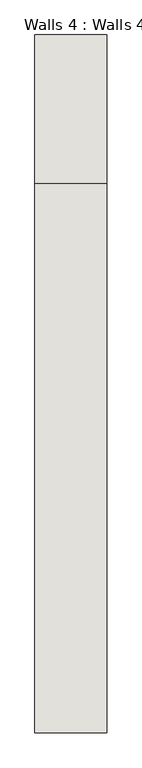
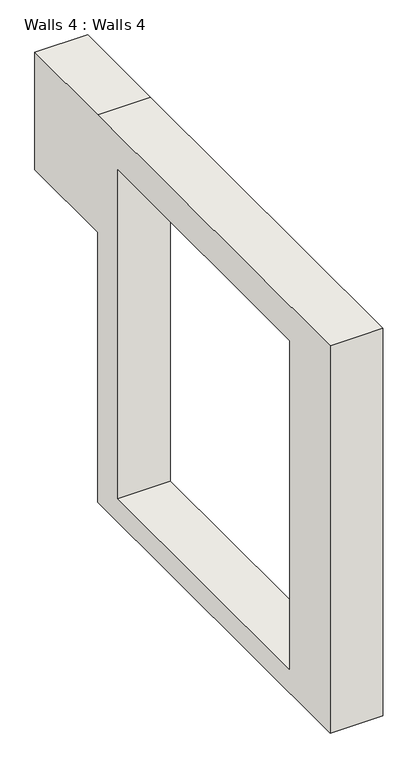
"""IFC4 building model written with IfcOpenShell, lengths in millimetres: wall geometry, Walls 4 : Walls 4."""

from ifc_helpers import new_model, si_unit, frame, origin, place, context, project, spatial, polyline, outline, extrude, source, transform, mapped, element, save


def walls_4_walls_4_aecb3609(model_context):
    return source(origin(), model_context, "Body", "SweptSolid", [
        extrude(outline(polyline([(10469.0609482, 7315.2), (11358.0609482, 7315.2), (11358.0609482, 6299.2), (10469.0609482, 6299.2), (10469.0609482, 3962.4), (7172.415375, 3962.4), (7172.415375, 7315.2), (10469.0609482, 7315.2)]), holes=[polyline([(7748.6597172, 7010.4), (7748.6597172, 4163.611227), (10187.0597172, 4163.611227), (10187.0597172, 7010.4), (7748.6597172, 7010.4)])]), frame((-12218.0932708, 0.0, 0.0), z_axis=(1.0, 0.0, 0.0), x_axis=(0.0, 1.0, 0.0)), (0.0, 0.0, 1.0), 431.8),
    ])


if __name__ == "__main__":
    model = new_model("IFC4")
    model_context = context("Model", 3, world=origin())
    ifc_project = project(units=[si_unit("LENGTHUNIT", "METRE", prefix="MILLI")], contexts=[model_context])
    site = spatial("IfcSite", under=ifc_project)
    building = spatial("IfcBuilding", under=site)
    placement = place(None, origin())
    walls_4_walls_4_shape = walls_4_walls_4_aecb3609(model_context)
    element("IfcWall", 1, ObjectType="Walls 4 : Walls 4", at=placement, inside=building, context=model_context, shape_type="MappedRepresentation", body=[
        mapped(walls_4_walls_4_shape, transform((0.0, 0.0, 0.0), x_axis=(1.0, 0.0, 0.0), y_axis=(0.0, 1.0, 0.0), z_axis=(0.0, 0.0, 1.0))),
    ])
    save(model, "model.ifc")

# Revit data of these elements
# Element 1 (IfcWall, "Walls 4 : Walls 4")
#   Materials on its faces: "Default Wall"
# Materials
#   "Default Wall": colour RGB 128 128 128, transparency 0
